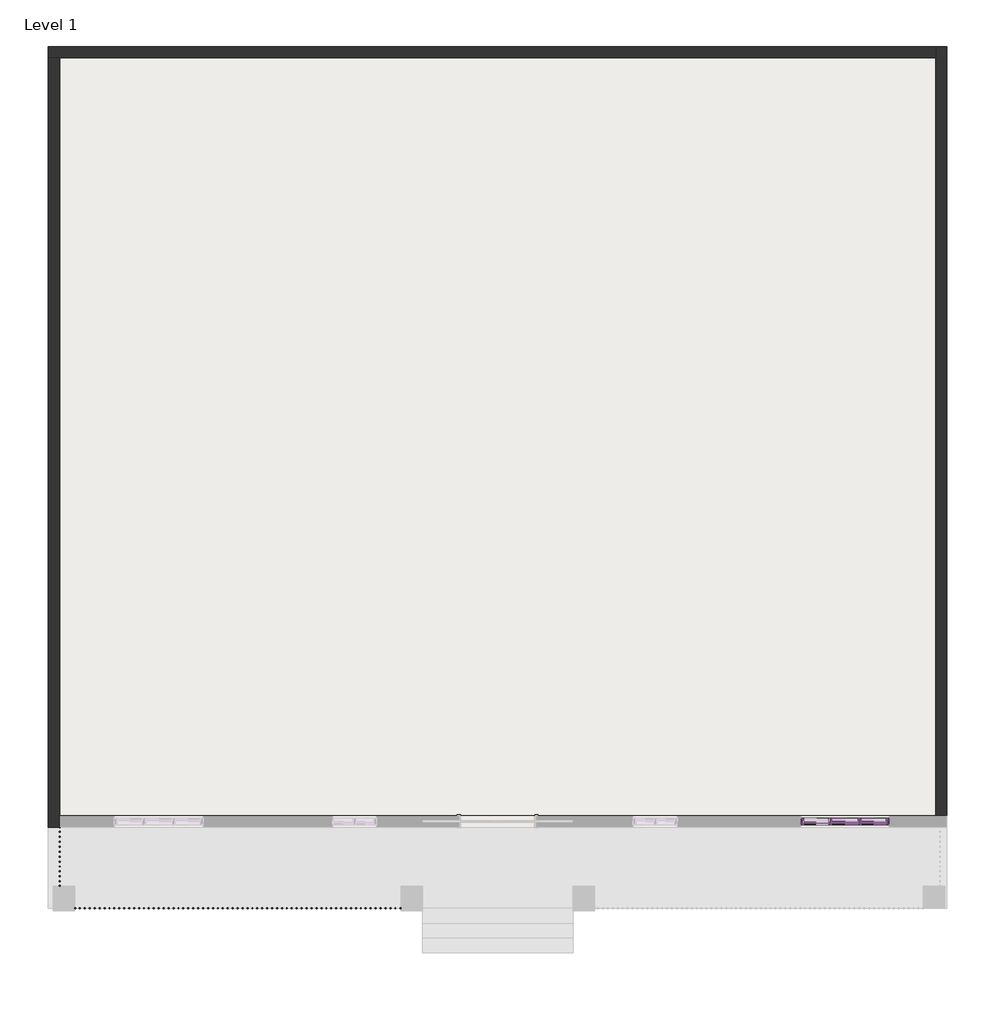
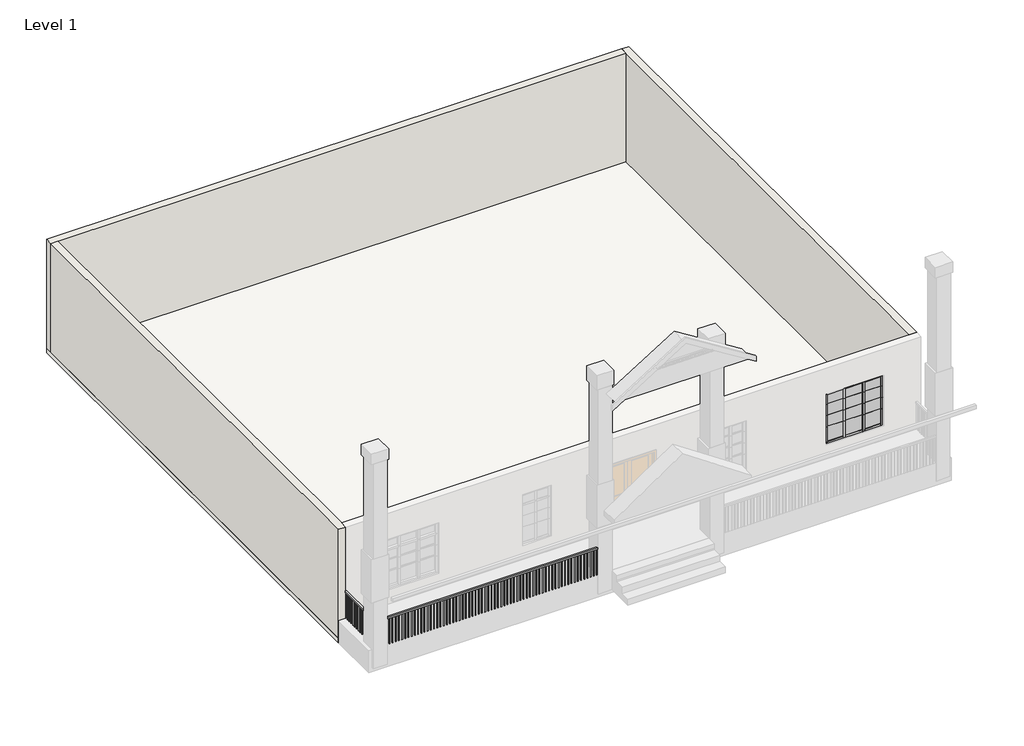
# One storey, part 2 of 3: 27 members, 12 plates, 3 walls, 2 railings, 1 slab.
"""IFC4 building model written with IfcOpenShell, lengths in millimetres."""

from ifc_helpers import new_model, si_unit, frame, origin, place, context, project, spatial, polyline, outline, extrude, faceted_brep, transform, mapped, element, save
from components import member_9625144b, member_80fbcd94, member_0b7646a3, member_bc554fa6, member_a980948f, member_03a502dc, member_dfe75557, member_50cacee6, system_panel_glazed_6026b5c4, system_panel_glazed_0f474f61, system_panel_glazed_969e6b50, system_panel_glazed_86de8a05, system_panel_glazed_f6df7fa7, system_panel_glazed_f12bf2b5

model = new_model("IFC4")

# Units and contexts
model_context = context("Model", 3, world=origin())
ifc_project = project(units=[si_unit("LENGTHUNIT", "METRE", prefix="MILLI")], contexts=[model_context])

# Site, building, storey
site = spatial("IfcSite", under=ifc_project)
building = spatial("IfcBuilding", under=site)
storey = spatial("IfcBuildingStorey", under=building, Name="Level 1", Elevation=0.0)

# Members
placement = place(None, origin())
member_shape = member_9625144b(model_context)
element("IfcMember", 1, ObjectType="Rectangular Mullion : 1\" Square", at=placement, inside=storey, context=model_context, shape_type="MappedRepresentation", body=[
    mapped(member_shape, transform((6987.2079341, -6986.1878342, 2006.6), x_axis=(0.0, 0.0, 1.0), y_axis=(0.0, 1.0, 0.0), z_axis=(-1.0, 0.0, 0.0))),
])
element("IfcMember", 2, ObjectType="Rectangular Mullion : 1\" Square", at=placement, inside=storey, context=model_context, shape_type="MappedRepresentation", body=[
    mapped(member_shape, transform((6987.2079341, -6986.1878342, 1625.6), x_axis=(0.0, 0.0, 1.0), y_axis=(0.0, 1.0, 0.0), z_axis=(-1.0, 0.0, 0.0))),
])
element("IfcMember", 3, ObjectType="Rectangular Mullion : 1\" Square", at=placement, inside=storey, context=model_context, shape_type="MappedRepresentation", body=[
    mapped(member_shape, transform((6987.2079341, -6986.1878342, 2387.6), x_axis=(0.0, 0.0, 1.0), y_axis=(0.0, 1.0, 0.0), z_axis=(-1.0, 0.0, 0.0))),
])
member_2_shape = member_80fbcd94(model_context)
element("IfcMember", 4, ObjectType="Rectangular Mullion : 1\" Square", at=placement, inside=storey, context=model_context, shape_type="MappedRepresentation", body=[
    mapped(member_2_shape, transform((6377.6079341, -6986.1878342, 2006.6), x_axis=(0.0, 0.0, 1.0), y_axis=(0.0, 1.0, 0.0), z_axis=(-1.0, 0.0, 0.0))),
])
element("IfcMember", 5, ObjectType="Rectangular Mullion : 1\" Square", at=placement, inside=storey, context=model_context, shape_type="MappedRepresentation", body=[
    mapped(member_2_shape, transform((6377.6079341, -6986.1878342, 1625.6), x_axis=(0.0, 0.0, 1.0), y_axis=(0.0, 1.0, 0.0), z_axis=(-1.0, 0.0, 0.0))),
])
element("IfcMember", 6, ObjectType="Rectangular Mullion : 1\" Square", at=placement, inside=storey, context=model_context, shape_type="MappedRepresentation", body=[
    mapped(member_2_shape, transform((6377.6079341, -6986.1878342, 2387.6), x_axis=(0.0, 0.0, 1.0), y_axis=(0.0, 1.0, 0.0), z_axis=(-1.0, 0.0, 0.0))),
])
member_3_shape = member_0b7646a3(model_context)
element("IfcMember", 7, ObjectType="Rectangular Mullion : 2.5\" x 5\" rectangular", at=placement, inside=storey, context=model_context, shape_type="MappedRepresentation", body=[
    mapped(member_3_shape, transform((6987.2079341, -6986.1878342, 2768.6), x_axis=(0.0, 0.0, 1.0), y_axis=(0.0, 1.0, 0.0), z_axis=(-1.0, 0.0, 0.0))),
])
element("IfcMember", 8, ObjectType="Rectangular Mullion : 2.5\" x 5\" rectangular", at=placement, inside=storey, context=model_context, shape_type="MappedRepresentation", body=[
    mapped(member_3_shape, transform((7501.5579341, -6986.1878342, 1066.8), x_axis=(0.0, 0.0, -1.0), y_axis=(0.0, 1.0, 0.0), z_axis=(1.0, 0.0, 0.0))),
])
element("IfcMember", 9, ObjectType="Rectangular Mullion : 2.5\" x 5\" rectangular", at=placement, inside=storey, context=model_context, shape_type="MappedRepresentation", body=[
    mapped(member_3_shape, transform((6314.1079341, -6986.1878342, 1066.8), x_axis=(0.0, 0.0, -1.0), y_axis=(0.0, 1.0, 0.0), z_axis=(1.0, 0.0, 0.0))),
])
member_4_shape = member_bc554fa6(model_context)
element("IfcMember", 10, ObjectType="Rectangular Mullion : 2.5\" x 5\" rectangular", at=placement, inside=storey, context=model_context, shape_type="MappedRepresentation", body=[
    mapped(member_4_shape, transform((6345.8579341, -6986.1878342, 1066.8), x_axis=(-1.0, 0.0, 0.0), y_axis=(0.0, 1.0, 0.0), z_axis=(0.0, 0.0, -1.0))),
])
element("IfcMember", 11, ObjectType="Rectangular Mullion : 2.5\" x 5\" rectangular", at=placement, inside=storey, context=model_context, shape_type="MappedRepresentation", body=[
    mapped(member_4_shape, transform((6955.4579341, -6986.1878342, 1066.8), x_axis=(-1.0, 0.0, 0.0), y_axis=(0.0, 1.0, 0.0), z_axis=(0.0, 0.0, -1.0))),
])
member_5_shape = member_a980948f(model_context)
element("IfcMember", 12, ObjectType="Rectangular Mullion : 2.5\" x 5\" rectangular", at=placement, inside=storey, context=model_context, shape_type="MappedRepresentation", body=[
    mapped(member_5_shape, transform((6923.7079341, -6986.1878342, 1066.8), x_axis=(0.0, 0.0, -1.0), y_axis=(0.0, 1.0, 0.0), z_axis=(1.0, 0.0, 0.0))),
])
element("IfcMember", 13, ObjectType="Rectangular Mullion : 2.5\" x 5\" rectangular", at=placement, inside=storey, context=model_context, shape_type="MappedRepresentation", body=[
    mapped(member_5_shape, transform((6377.6079341, -6986.1878342, 2768.6), x_axis=(0.0, 0.0, 1.0), y_axis=(0.0, 1.0, 0.0), z_axis=(-1.0, 0.0, 0.0))),
])
member_6_shape = member_03a502dc(model_context)
element("IfcMember", 14, ObjectType="Rectangular Mullion : 2.5\" x 5\" rectangular", at=placement, inside=storey, context=model_context, shape_type="MappedRepresentation", body=[
    mapped(member_6_shape, transform((6345.8579341, -6986.1878342, 2387.6), x_axis=(-1.0, 0.0, 0.0), y_axis=(0.0, 1.0, 0.0), z_axis=(0.0, 0.0, -1.0))),
])
element("IfcMember", 15, ObjectType="Rectangular Mullion : 2.5\" x 5\" rectangular", at=placement, inside=storey, context=model_context, shape_type="MappedRepresentation", body=[
    mapped(member_6_shape, transform((6955.4579341, -6986.1878342, 2387.6), x_axis=(-1.0, 0.0, 0.0), y_axis=(0.0, 1.0, 0.0), z_axis=(0.0, 0.0, -1.0))),
])
element("IfcMember", 16, ObjectType="Rectangular Mullion : 2.5\" x 5\" rectangular", at=placement, inside=storey, context=model_context, shape_type="MappedRepresentation", body=[
    mapped(member_6_shape, transform((6345.8579341, -6986.1878342, 2006.6), x_axis=(-1.0, 0.0, 0.0), y_axis=(0.0, 1.0, 0.0), z_axis=(0.0, 0.0, -1.0))),
])
element("IfcMember", 17, ObjectType="Rectangular Mullion : 2.5\" x 5\" rectangular", at=placement, inside=storey, context=model_context, shape_type="MappedRepresentation", body=[
    mapped(member_6_shape, transform((6345.8579341, -6986.1878342, 1625.6), x_axis=(-1.0, 0.0, 0.0), y_axis=(0.0, 1.0, 0.0), z_axis=(0.0, 0.0, -1.0))),
])
element("IfcMember", 18, ObjectType="Rectangular Mullion : 2.5\" x 5\" rectangular", at=placement, inside=storey, context=model_context, shape_type="MappedRepresentation", body=[
    mapped(member_6_shape, transform((6955.4579341, -6986.1878342, 2006.6), x_axis=(-1.0, 0.0, 0.0), y_axis=(0.0, 1.0, 0.0), z_axis=(0.0, 0.0, -1.0))),
])
element("IfcMember", 19, ObjectType="Rectangular Mullion : 2.5\" x 5\" rectangular", at=placement, inside=storey, context=model_context, shape_type="MappedRepresentation", body=[
    mapped(member_6_shape, transform((6955.4579341, -6986.1878342, 1625.6), x_axis=(-1.0, 0.0, 0.0), y_axis=(0.0, 1.0, 0.0), z_axis=(0.0, 0.0, -1.0))),
])
member_7_shape = member_dfe75557(model_context)
element("IfcMember", 20, ObjectType="Rectangular Mullion : 2.5\" x 5\" rectangular", at=placement, inside=storey, context=model_context, shape_type="MappedRepresentation", body=[
    mapped(member_7_shape, transform((7565.0579341, -6986.1878342, 2768.6), x_axis=(1.0, 0.0, 0.0), y_axis=(0.0, 1.0, 0.0), z_axis=(0.0, 0.0, 1.0))),
])
member_8_shape = member_50cacee6(model_context)
element("IfcMember", 21, ObjectType="Rectangular Mullion : 2.5\" x 5\" rectangular", at=placement, inside=storey, context=model_context, shape_type="MappedRepresentation", body=[
    mapped(member_8_shape, transform((5736.2579341, -6986.1878342, 1066.8), x_axis=(-1.0, 0.0, 0.0), y_axis=(0.0, 1.0, 0.0), z_axis=(0.0, 0.0, -1.0))),
])
element("IfcMember", 22, ObjectType="Rectangular Mullion : 2.5\" x 5\" rectangular", at=placement, inside=storey, context=model_context, shape_type="MappedRepresentation", body=[
    mapped(member_7_shape, transform((5736.2579341, -6986.1878342, 2387.6), x_axis=(-1.0, 0.0, 0.0), y_axis=(0.0, 1.0, 0.0), z_axis=(0.0, 0.0, -1.0))),
])
element("IfcMember", 23, ObjectType="Rectangular Mullion : 2.5\" x 5\" rectangular", at=placement, inside=storey, context=model_context, shape_type="MappedRepresentation", body=[
    mapped(member_7_shape, transform((5736.2579341, -6986.1878342, 2006.6), x_axis=(-1.0, 0.0, 0.0), y_axis=(0.0, 1.0, 0.0), z_axis=(0.0, 0.0, -1.0))),
])
element("IfcMember", 24, ObjectType="Rectangular Mullion : 2.5\" x 5\" rectangular", at=placement, inside=storey, context=model_context, shape_type="MappedRepresentation", body=[
    mapped(member_7_shape, transform((5736.2579341, -6986.1878342, 1625.6), x_axis=(-1.0, 0.0, 0.0), y_axis=(0.0, 1.0, 0.0), z_axis=(0.0, 0.0, -1.0))),
])
element("IfcMember", 25, ObjectType="Rectangular Mullion : 2.5\" x 5\" rectangular", at=placement, inside=storey, context=model_context, shape_type="MappedRepresentation", body=[
    mapped(member_7_shape, transform((7565.0579341, -6986.1878342, 2387.6), x_axis=(1.0, 0.0, 0.0), y_axis=(0.0, 1.0, 0.0), z_axis=(0.0, 0.0, 1.0))),
])
element("IfcMember", 26, ObjectType="Rectangular Mullion : 2.5\" x 5\" rectangular", at=placement, inside=storey, context=model_context, shape_type="MappedRepresentation", body=[
    mapped(member_7_shape, transform((7565.0579341, -6986.1878342, 2006.6), x_axis=(1.0, 0.0, 0.0), y_axis=(0.0, 1.0, 0.0), z_axis=(0.0, 0.0, 1.0))),
])
element("IfcMember", 27, ObjectType="Rectangular Mullion : 2.5\" x 5\" rectangular", at=placement, inside=storey, context=model_context, shape_type="MappedRepresentation", body=[
    mapped(member_8_shape, transform((7565.0579341, -6986.1878342, 1625.6), x_axis=(1.0, 0.0, 0.0), y_axis=(0.0, 1.0, 0.0), z_axis=(0.0, 0.0, 1.0))),
])

# Plates
system_panel_glazed_shape = system_panel_glazed_6026b5c4(model_context)
element("IfcPlate", 28, ObjectType="System Panel : Glazed", at=placement, inside=storey, context=model_context, shape_type="MappedRepresentation", body=[
    mapped(system_panel_glazed_shape, transform((7244.3829341, -6986.1878342, 1130.3), x_axis=(-1.0, 0.0, 0.0), y_axis=(0.0, -1.0, 0.0), z_axis=(0.0, 0.0, 1.0))),
])
element("IfcPlate", 29, ObjectType="System Panel : Glazed", at=placement, inside=storey, context=model_context, shape_type="MappedRepresentation", body=[
    mapped(system_panel_glazed_shape, transform((6056.9329341, -6986.1878342, 1130.3), x_axis=(-1.0, 0.0, 0.0), y_axis=(0.0, -1.0, 0.0), z_axis=(0.0, 0.0, 1.0))),
])
system_panel_glazed_2_shape = system_panel_glazed_0f474f61(model_context)
element("IfcPlate", 30, ObjectType="System Panel : Glazed", at=placement, inside=storey, context=model_context, shape_type="MappedRepresentation", body=[
    mapped(system_panel_glazed_2_shape, transform((6650.6579341, -6986.1878342, 1130.3), x_axis=(-1.0, 0.0, 0.0), y_axis=(0.0, -1.0, 0.0), z_axis=(0.0, 0.0, 1.0))),
])
system_panel_glazed_3_shape = system_panel_glazed_969e6b50(model_context)
element("IfcPlate", 31, ObjectType="System Panel : Glazed", at=placement, inside=storey, context=model_context, shape_type="MappedRepresentation", body=[
    mapped(system_panel_glazed_3_shape, transform((7244.3829341, -6986.1878342, 2006.6), x_axis=(-1.0, 0.0, 0.0), y_axis=(0.0, -1.0, 0.0), z_axis=(0.0, 0.0, 1.0))),
])
element("IfcPlate", 32, ObjectType="System Panel : Glazed", at=placement, inside=storey, context=model_context, shape_type="MappedRepresentation", body=[
    mapped(system_panel_glazed_3_shape, transform((6056.9329341, -6986.1878342, 2006.6), x_axis=(-1.0, 0.0, 0.0), y_axis=(0.0, -1.0, 0.0), z_axis=(0.0, 0.0, 1.0))),
])
element("IfcPlate", 33, ObjectType="System Panel : Glazed", at=placement, inside=storey, context=model_context, shape_type="MappedRepresentation", body=[
    mapped(system_panel_glazed_3_shape, transform((7244.3829341, -6986.1878342, 1625.6), x_axis=(-1.0, 0.0, 0.0), y_axis=(0.0, -1.0, 0.0), z_axis=(0.0, 0.0, 1.0))),
])
element("IfcPlate", 34, ObjectType="System Panel : Glazed", at=placement, inside=storey, context=model_context, shape_type="MappedRepresentation", body=[
    mapped(system_panel_glazed_3_shape, transform((6056.9329341, -6986.1878342, 1625.6), x_axis=(-1.0, 0.0, 0.0), y_axis=(0.0, -1.0, 0.0), z_axis=(0.0, 0.0, 1.0))),
])
system_panel_glazed_4_shape = system_panel_glazed_86de8a05(model_context)
element("IfcPlate", 35, ObjectType="System Panel : Glazed", at=placement, inside=storey, context=model_context, shape_type="MappedRepresentation", body=[
    mapped(system_panel_glazed_4_shape, transform((6650.6579341, -6986.1878342, 2006.6), x_axis=(-1.0, 0.0, 0.0), y_axis=(0.0, -1.0, 0.0), z_axis=(0.0, 0.0, 1.0))),
])
element("IfcPlate", 36, ObjectType="System Panel : Glazed", at=placement, inside=storey, context=model_context, shape_type="MappedRepresentation", body=[
    mapped(system_panel_glazed_4_shape, transform((6650.6579341, -6986.1878342, 1625.6), x_axis=(-1.0, 0.0, 0.0), y_axis=(0.0, -1.0, 0.0), z_axis=(0.0, 0.0, 1.0))),
])
system_panel_glazed_5_shape = system_panel_glazed_f6df7fa7(model_context)
element("IfcPlate", 37, ObjectType="System Panel : Glazed", at=placement, inside=storey, context=model_context, shape_type="MappedRepresentation", body=[
    mapped(system_panel_glazed_5_shape, transform((7244.3829341, -6986.1878342, 2387.6), x_axis=(-1.0, 0.0, 0.0), y_axis=(0.0, -1.0, 0.0), z_axis=(0.0, 0.0, 1.0))),
])
element("IfcPlate", 38, ObjectType="System Panel : Glazed", at=placement, inside=storey, context=model_context, shape_type="MappedRepresentation", body=[
    mapped(system_panel_glazed_5_shape, transform((6056.9329341, -6986.1878342, 2387.6), x_axis=(-1.0, 0.0, 0.0), y_axis=(0.0, -1.0, 0.0), z_axis=(0.0, 0.0, 1.0))),
])
system_panel_glazed_6_shape = system_panel_glazed_f12bf2b5(model_context)
element("IfcPlate", 39, ObjectType="System Panel : Glazed", at=placement, inside=storey, context=model_context, shape_type="MappedRepresentation", body=[
    mapped(system_panel_glazed_6_shape, transform((6650.6579341, -6986.1878342, 2387.6), x_axis=(-1.0, 0.0, 0.0), y_axis=(0.0, -1.0, 0.0), z_axis=(0.0, 0.0, 1.0))),
])

# Railings
element("IfcRailing", 40, ObjectType="Handrail - Rectangular", at=placement, inside=storey, context=model_context, shape_type="SweptSolid", body=[
    extrude(outline(polyline([(-9224.3420659, -8800.5902135), (-9224.3420659, -8749.7902135), (-2506.0420659, -8749.7902135), (-2506.0420659, -8800.5902135), (-9224.3420659, -8800.5902135)])), frame((0.0, 0.0, 1473.2), z_axis=(0.0, 0.0, 1.0), x_axis=(1.0, 0.0, 0.0)), (0.0, 0.0, 1.0), 50.8),
    extrude(outline(polyline([(-2528.2670659, -8784.7152135), (-2528.2670659, -8765.6652135), (-2509.2170659, -8765.6652135), (-2509.2170659, -8784.7152135), (-2528.2670659, -8784.7152135)])), frame((0.0, 0.0, 609.6), z_axis=(0.0, 0.0, 1.0), x_axis=(1.0, 0.0, 0.0)), (0.0, 0.0, 1.0), 863.6),
    extrude(outline(polyline([(-2629.8670659, -8784.7152135), (-2629.8670659, -8765.6652135), (-2610.8170659, -8765.6652135), (-2610.8170659, -8784.7152135), (-2629.8670659, -8784.7152135)])), frame((0.0, 0.0, 609.6), z_axis=(0.0, 0.0, 1.0), x_axis=(1.0, 0.0, 0.0)), (0.0, 0.0, 1.0), 863.6),
    extrude(outline(polyline([(-2731.4670659, -8784.7152135), (-2731.4670659, -8765.6652135), (-2712.4170659, -8765.6652135), (-2712.4170659, -8784.7152135), (-2731.4670659, -8784.7152135)])), frame((0.0, 0.0, 609.6), z_axis=(0.0, 0.0, 1.0), x_axis=(1.0, 0.0, 0.0)), (0.0, 0.0, 1.0), 863.6),
    extrude(outline(polyline([(-2833.0670659, -8784.7152135), (-2833.0670659, -8765.6652135), (-2814.0170659, -8765.6652135), (-2814.0170659, -8784.7152135), (-2833.0670659, -8784.7152135)])), frame((0.0, 0.0, 609.6), z_axis=(0.0, 0.0, 1.0), x_axis=(1.0, 0.0, 0.0)), (0.0, 0.0, 1.0), 863.6),
    extrude(outline(polyline([(-2934.6670659, -8784.7152135), (-2934.6670659, -8765.6652135), (-2915.6170659, -8765.6652135), (-2915.6170659, -8784.7152135), (-2934.6670659, -8784.7152135)])), frame((0.0, 0.0, 609.6), z_axis=(0.0, 0.0, 1.0), x_axis=(1.0, 0.0, 0.0)), (0.0, 0.0, 1.0), 863.6),
    extrude(outline(polyline([(-3036.2670659, -8784.7152135), (-3036.2670659, -8765.6652135), (-3017.2170659, -8765.6652135), (-3017.2170659, -8784.7152135), (-3036.2670659, -8784.7152135)])), frame((0.0, 0.0, 609.6), z_axis=(0.0, 0.0, 1.0), x_axis=(1.0, 0.0, 0.0)), (0.0, 0.0, 1.0), 863.6),
    extrude(outline(polyline([(-3137.8670659, -8784.7152135), (-3137.8670659, -8765.6652135), (-3118.8170659, -8765.6652135), (-3118.8170659, -8784.7152135), (-3137.8670659, -8784.7152135)])), frame((0.0, 0.0, 609.6), z_axis=(0.0, 0.0, 1.0), x_axis=(1.0, 0.0, 0.0)), (0.0, 0.0, 1.0), 863.6),
    extrude(outline(polyline([(-3239.4670659, -8784.7152135), (-3239.4670659, -8765.6652135), (-3220.4170659, -8765.6652135), (-3220.4170659, -8784.7152135), (-3239.4670659, -8784.7152135)])), frame((0.0, 0.0, 609.6), z_axis=(0.0, 0.0, 1.0), x_axis=(1.0, 0.0, 0.0)), (0.0, 0.0, 1.0), 863.6),
    extrude(outline(polyline([(-3341.0670659, -8784.7152135), (-3341.0670659, -8765.6652135), (-3322.0170659, -8765.6652135), (-3322.0170659, -8784.7152135), (-3341.0670659, -8784.7152135)])), frame((0.0, 0.0, 609.6), z_axis=(0.0, 0.0, 1.0), x_axis=(1.0, 0.0, 0.0)), (0.0, 0.0, 1.0), 863.6),
    extrude(outline(polyline([(-3442.6670659, -8784.7152135), (-3442.6670659, -8765.6652135), (-3423.6170659, -8765.6652135), (-3423.6170659, -8784.7152135), (-3442.6670659, -8784.7152135)])), frame((0.0, 0.0, 609.6), z_axis=(0.0, 0.0, 1.0), x_axis=(1.0, 0.0, 0.0)), (0.0, 0.0, 1.0), 863.6),
    extrude(outline(polyline([(-3544.2670659, -8784.7152135), (-3544.2670659, -8765.6652135), (-3525.2170659, -8765.6652135), (-3525.2170659, -8784.7152135), (-3544.2670659, -8784.7152135)])), frame((0.0, 0.0, 609.6), z_axis=(0.0, 0.0, 1.0), x_axis=(1.0, 0.0, 0.0)), (0.0, 0.0, 1.0), 863.6),
    extrude(outline(polyline([(-3645.8670659, -8784.7152135), (-3645.8670659, -8765.6652135), (-3626.8170659, -8765.6652135), (-3626.8170659, -8784.7152135), (-3645.8670659, -8784.7152135)])), frame((0.0, 0.0, 609.6), z_axis=(0.0, 0.0, 1.0), x_axis=(1.0, 0.0, 0.0)), (0.0, 0.0, 1.0), 863.6),
    extrude(outline(polyline([(-3747.4670659, -8784.7152135), (-3747.4670659, -8765.6652135), (-3728.4170659, -8765.6652135), (-3728.4170659, -8784.7152135), (-3747.4670659, -8784.7152135)])), frame((0.0, 0.0, 609.6), z_axis=(0.0, 0.0, 1.0), x_axis=(1.0, 0.0, 0.0)), (0.0, 0.0, 1.0), 863.6),
    extrude(outline(polyline([(-3849.0670659, -8784.7152135), (-3849.0670659, -8765.6652135), (-3830.0170659, -8765.6652135), (-3830.0170659, -8784.7152135), (-3849.0670659, -8784.7152135)])), frame((0.0, 0.0, 609.6), z_axis=(0.0, 0.0, 1.0), x_axis=(1.0, 0.0, 0.0)), (0.0, 0.0, 1.0), 863.6),
    extrude(outline(polyline([(-3950.6670659, -8784.7152135), (-3950.6670659, -8765.6652135), (-3931.6170659, -8765.6652135), (-3931.6170659, -8784.7152135), (-3950.6670659, -8784.7152135)])), frame((0.0, 0.0, 609.6), z_axis=(0.0, 0.0, 1.0), x_axis=(1.0, 0.0, 0.0)), (0.0, 0.0, 1.0), 863.6),
    extrude(outline(polyline([(-4052.2670659, -8784.7152135), (-4052.2670659, -8765.6652135), (-4033.2170659, -8765.6652135), (-4033.2170659, -8784.7152135), (-4052.2670659, -8784.7152135)])), frame((0.0, 0.0, 609.6), z_axis=(0.0, 0.0, 1.0), x_axis=(1.0, 0.0, 0.0)), (0.0, 0.0, 1.0), 863.6),
    extrude(outline(polyline([(-4153.8670659, -8784.7152135), (-4153.8670659, -8765.6652135), (-4134.8170659, -8765.6652135), (-4134.8170659, -8784.7152135), (-4153.8670659, -8784.7152135)])), frame((0.0, 0.0, 609.6), z_axis=(0.0, 0.0, 1.0), x_axis=(1.0, 0.0, 0.0)), (0.0, 0.0, 1.0), 863.6),
    extrude(outline(polyline([(-4255.4670659, -8784.7152135), (-4255.4670659, -8765.6652135), (-4236.4170659, -8765.6652135), (-4236.4170659, -8784.7152135), (-4255.4670659, -8784.7152135)])), frame((0.0, 0.0, 609.6), z_axis=(0.0, 0.0, 1.0), x_axis=(1.0, 0.0, 0.0)), (0.0, 0.0, 1.0), 863.6),
    extrude(outline(polyline([(-4357.0670659, -8784.7152135), (-4357.0670659, -8765.6652135), (-4338.0170659, -8765.6652135), (-4338.0170659, -8784.7152135), (-4357.0670659, -8784.7152135)])), frame((0.0, 0.0, 609.6), z_axis=(0.0, 0.0, 1.0), x_axis=(1.0, 0.0, 0.0)), (0.0, 0.0, 1.0), 863.6),
    extrude(outline(polyline([(-4458.6670659, -8784.7152135), (-4458.6670659, -8765.6652135), (-4439.6170659, -8765.6652135), (-4439.6170659, -8784.7152135), (-4458.6670659, -8784.7152135)])), frame((0.0, 0.0, 609.6), z_axis=(0.0, 0.0, 1.0), x_axis=(1.0, 0.0, 0.0)), (0.0, 0.0, 1.0), 863.6),
    extrude(outline(polyline([(-4560.2670659, -8784.7152135), (-4560.2670659, -8765.6652135), (-4541.2170659, -8765.6652135), (-4541.2170659, -8784.7152135), (-4560.2670659, -8784.7152135)])), frame((0.0, 0.0, 609.6), z_axis=(0.0, 0.0, 1.0), x_axis=(1.0, 0.0, 0.0)), (0.0, 0.0, 1.0), 863.6),
    extrude(outline(polyline([(-4661.8670659, -8784.7152135), (-4661.8670659, -8765.6652135), (-4642.8170659, -8765.6652135), (-4642.8170659, -8784.7152135), (-4661.8670659, -8784.7152135)])), frame((0.0, 0.0, 609.6), z_axis=(0.0, 0.0, 1.0), x_axis=(1.0, 0.0, 0.0)), (0.0, 0.0, 1.0), 863.6),
    extrude(outline(polyline([(-4763.4670659, -8784.7152135), (-4763.4670659, -8765.6652135), (-4744.4170659, -8765.6652135), (-4744.4170659, -8784.7152135), (-4763.4670659, -8784.7152135)])), frame((0.0, 0.0, 609.6), z_axis=(0.0, 0.0, 1.0), x_axis=(1.0, 0.0, 0.0)), (0.0, 0.0, 1.0), 863.6),
    extrude(outline(polyline([(-4865.0670659, -8784.7152135), (-4865.0670659, -8765.6652135), (-4846.0170659, -8765.6652135), (-4846.0170659, -8784.7152135), (-4865.0670659, -8784.7152135)])), frame((0.0, 0.0, 609.6), z_axis=(0.0, 0.0, 1.0), x_axis=(1.0, 0.0, 0.0)), (0.0, 0.0, 1.0), 863.6),
    extrude(outline(polyline([(-4966.6670659, -8784.7152135), (-4966.6670659, -8765.6652135), (-4947.6170659, -8765.6652135), (-4947.6170659, -8784.7152135), (-4966.6670659, -8784.7152135)])), frame((0.0, 0.0, 609.6), z_axis=(0.0, 0.0, 1.0), x_axis=(1.0, 0.0, 0.0)), (0.0, 0.0, 1.0), 863.6),
    extrude(outline(polyline([(-5068.2670659, -8784.7152135), (-5068.2670659, -8765.6652135), (-5049.2170659, -8765.6652135), (-5049.2170659, -8784.7152135), (-5068.2670659, -8784.7152135)])), frame((0.0, 0.0, 609.6), z_axis=(0.0, 0.0, 1.0), x_axis=(1.0, 0.0, 0.0)), (0.0, 0.0, 1.0), 863.6),
    extrude(outline(polyline([(-5169.8670659, -8784.7152135), (-5169.8670659, -8765.6652135), (-5150.8170659, -8765.6652135), (-5150.8170659, -8784.7152135), (-5169.8670659, -8784.7152135)])), frame((0.0, 0.0, 609.6), z_axis=(0.0, 0.0, 1.0), x_axis=(1.0, 0.0, 0.0)), (0.0, 0.0, 1.0), 863.6),
    extrude(outline(polyline([(-5271.4670659, -8784.7152135), (-5271.4670659, -8765.6652135), (-5252.4170659, -8765.6652135), (-5252.4170659, -8784.7152135), (-5271.4670659, -8784.7152135)])), frame((0.0, 0.0, 609.6), z_axis=(0.0, 0.0, 1.0), x_axis=(1.0, 0.0, 0.0)), (0.0, 0.0, 1.0), 863.6),
    extrude(outline(polyline([(-5373.0670659, -8784.7152135), (-5373.0670659, -8765.6652135), (-5354.0170659, -8765.6652135), (-5354.0170659, -8784.7152135), (-5373.0670659, -8784.7152135)])), frame((0.0, 0.0, 609.6), z_axis=(0.0, 0.0, 1.0), x_axis=(1.0, 0.0, 0.0)), (0.0, 0.0, 1.0), 863.6),
    extrude(outline(polyline([(-5474.6670659, -8784.7152135), (-5474.6670659, -8765.6652135), (-5455.6170659, -8765.6652135), (-5455.6170659, -8784.7152135), (-5474.6670659, -8784.7152135)])), frame((0.0, 0.0, 609.6), z_axis=(0.0, 0.0, 1.0), x_axis=(1.0, 0.0, 0.0)), (0.0, 0.0, 1.0), 863.6),
    extrude(outline(polyline([(-5576.2670659, -8784.7152135), (-5576.2670659, -8765.6652135), (-5557.2170659, -8765.6652135), (-5557.2170659, -8784.7152135), (-5576.2670659, -8784.7152135)])), frame((0.0, 0.0, 609.6), z_axis=(0.0, 0.0, 1.0), x_axis=(1.0, 0.0, 0.0)), (0.0, 0.0, 1.0), 863.6),
    extrude(outline(polyline([(-5677.8670659, -8784.7152135), (-5677.8670659, -8765.6652135), (-5658.8170659, -8765.6652135), (-5658.8170659, -8784.7152135), (-5677.8670659, -8784.7152135)])), frame((0.0, 0.0, 609.6), z_axis=(0.0, 0.0, 1.0), x_axis=(1.0, 0.0, 0.0)), (0.0, 0.0, 1.0), 863.6),
    extrude(outline(polyline([(-5779.4670659, -8784.7152135), (-5779.4670659, -8765.6652135), (-5760.4170659, -8765.6652135), (-5760.4170659, -8784.7152135), (-5779.4670659, -8784.7152135)])), frame((0.0, 0.0, 609.6), z_axis=(0.0, 0.0, 1.0), x_axis=(1.0, 0.0, 0.0)), (0.0, 0.0, 1.0), 863.6),
    extrude(outline(polyline([(-5881.0670659, -8784.7152135), (-5881.0670659, -8765.6652135), (-5862.0170659, -8765.6652135), (-5862.0170659, -8784.7152135), (-5881.0670659, -8784.7152135)])), frame((0.0, 0.0, 609.6), z_axis=(0.0, 0.0, 1.0), x_axis=(1.0, 0.0, 0.0)), (0.0, 0.0, 1.0), 863.6),
    extrude(outline(polyline([(-5982.6670659, -8784.7152135), (-5982.6670659, -8765.6652135), (-5963.6170659, -8765.6652135), (-5963.6170659, -8784.7152135), (-5982.6670659, -8784.7152135)])), frame((0.0, 0.0, 609.6), z_axis=(0.0, 0.0, 1.0), x_axis=(1.0, 0.0, 0.0)), (0.0, 0.0, 1.0), 863.6),
    extrude(outline(polyline([(-6084.2670659, -8784.7152135), (-6084.2670659, -8765.6652135), (-6065.2170659, -8765.6652135), (-6065.2170659, -8784.7152135), (-6084.2670659, -8784.7152135)])), frame((0.0, 0.0, 609.6), z_axis=(0.0, 0.0, 1.0), x_axis=(1.0, 0.0, 0.0)), (0.0, 0.0, 1.0), 863.6),
    extrude(outline(polyline([(-6185.8670659, -8784.7152135), (-6185.8670659, -8765.6652135), (-6166.8170659, -8765.6652135), (-6166.8170659, -8784.7152135), (-6185.8670659, -8784.7152135)])), frame((0.0, 0.0, 609.6), z_axis=(0.0, 0.0, 1.0), x_axis=(1.0, 0.0, 0.0)), (0.0, 0.0, 1.0), 863.6),
    extrude(outline(polyline([(-6287.4670659, -8784.7152135), (-6287.4670659, -8765.6652135), (-6268.4170659, -8765.6652135), (-6268.4170659, -8784.7152135), (-6287.4670659, -8784.7152135)])), frame((0.0, 0.0, 609.6), z_axis=(0.0, 0.0, 1.0), x_axis=(1.0, 0.0, 0.0)), (0.0, 0.0, 1.0), 863.6),
    extrude(outline(polyline([(-6389.0670659, -8784.7152135), (-6389.0670659, -8765.6652135), (-6370.0170659, -8765.6652135), (-6370.0170659, -8784.7152135), (-6389.0670659, -8784.7152135)])), frame((0.0, 0.0, 609.6), z_axis=(0.0, 0.0, 1.0), x_axis=(1.0, 0.0, 0.0)), (0.0, 0.0, 1.0), 863.6),
    extrude(outline(polyline([(-6490.6670659, -8784.7152135), (-6490.6670659, -8765.6652135), (-6471.6170659, -8765.6652135), (-6471.6170659, -8784.7152135), (-6490.6670659, -8784.7152135)])), frame((0.0, 0.0, 609.6), z_axis=(0.0, 0.0, 1.0), x_axis=(1.0, 0.0, 0.0)), (0.0, 0.0, 1.0), 863.6),
    extrude(outline(polyline([(-6592.2670659, -8784.7152135), (-6592.2670659, -8765.6652135), (-6573.2170659, -8765.6652135), (-6573.2170659, -8784.7152135), (-6592.2670659, -8784.7152135)])), frame((0.0, 0.0, 609.6), z_axis=(0.0, 0.0, 1.0), x_axis=(1.0, 0.0, 0.0)), (0.0, 0.0, 1.0), 863.6),
    extrude(outline(polyline([(-6693.8670659, -8784.7152135), (-6693.8670659, -8765.6652135), (-6674.8170659, -8765.6652135), (-6674.8170659, -8784.7152135), (-6693.8670659, -8784.7152135)])), frame((0.0, 0.0, 609.6), z_axis=(0.0, 0.0, 1.0), x_axis=(1.0, 0.0, 0.0)), (0.0, 0.0, 1.0), 863.6),
    extrude(outline(polyline([(-6795.4670659, -8784.7152135), (-6795.4670659, -8765.6652135), (-6776.4170659, -8765.6652135), (-6776.4170659, -8784.7152135), (-6795.4670659, -8784.7152135)])), frame((0.0, 0.0, 609.6), z_axis=(0.0, 0.0, 1.0), x_axis=(1.0, 0.0, 0.0)), (0.0, 0.0, 1.0), 863.6),
    extrude(outline(polyline([(-6897.0670659, -8784.7152135), (-6897.0670659, -8765.6652135), (-6878.0170659, -8765.6652135), (-6878.0170659, -8784.7152135), (-6897.0670659, -8784.7152135)])), frame((0.0, 0.0, 609.6), z_axis=(0.0, 0.0, 1.0), x_axis=(1.0, 0.0, 0.0)), (0.0, 0.0, 1.0), 863.6),
    extrude(outline(polyline([(-6998.6670659, -8784.7152135), (-6998.6670659, -8765.6652135), (-6979.6170659, -8765.6652135), (-6979.6170659, -8784.7152135), (-6998.6670659, -8784.7152135)])), frame((0.0, 0.0, 609.6), z_axis=(0.0, 0.0, 1.0), x_axis=(1.0, 0.0, 0.0)), (0.0, 0.0, 1.0), 863.6),
    extrude(outline(polyline([(-7100.2670659, -8784.7152135), (-7100.2670659, -8765.6652135), (-7081.2170659, -8765.6652135), (-7081.2170659, -8784.7152135), (-7100.2670659, -8784.7152135)])), frame((0.0, 0.0, 609.6), z_axis=(0.0, 0.0, 1.0), x_axis=(1.0, 0.0, 0.0)), (0.0, 0.0, 1.0), 863.6),
    extrude(outline(polyline([(-7201.8670659, -8784.7152135), (-7201.8670659, -8765.6652135), (-7182.8170659, -8765.6652135), (-7182.8170659, -8784.7152135), (-7201.8670659, -8784.7152135)])), frame((0.0, 0.0, 609.6), z_axis=(0.0, 0.0, 1.0), x_axis=(1.0, 0.0, 0.0)), (0.0, 0.0, 1.0), 863.6),
    extrude(outline(polyline([(-7303.4670659, -8784.7152135), (-7303.4670659, -8765.6652135), (-7284.4170659, -8765.6652135), (-7284.4170659, -8784.7152135), (-7303.4670659, -8784.7152135)])), frame((0.0, 0.0, 609.6), z_axis=(0.0, 0.0, 1.0), x_axis=(1.0, 0.0, 0.0)), (0.0, 0.0, 1.0), 863.6),
    extrude(outline(polyline([(-7405.0670659, -8784.7152135), (-7405.0670659, -8765.6652135), (-7386.0170659, -8765.6652135), (-7386.0170659, -8784.7152135), (-7405.0670659, -8784.7152135)])), frame((0.0, 0.0, 609.6), z_axis=(0.0, 0.0, 1.0), x_axis=(1.0, 0.0, 0.0)), (0.0, 0.0, 1.0), 863.6),
    extrude(outline(polyline([(-7506.6670659, -8784.7152135), (-7506.6670659, -8765.6652135), (-7487.6170659, -8765.6652135), (-7487.6170659, -8784.7152135), (-7506.6670659, -8784.7152135)])), frame((0.0, 0.0, 609.6), z_axis=(0.0, 0.0, 1.0), x_axis=(1.0, 0.0, 0.0)), (0.0, 0.0, 1.0), 863.6),
    extrude(outline(polyline([(-7608.2670659, -8784.7152135), (-7608.2670659, -8765.6652135), (-7589.2170659, -8765.6652135), (-7589.2170659, -8784.7152135), (-7608.2670659, -8784.7152135)])), frame((0.0, 0.0, 609.6), z_axis=(0.0, 0.0, 1.0), x_axis=(1.0, 0.0, 0.0)), (0.0, 0.0, 1.0), 863.6),
    extrude(outline(polyline([(-7709.8670659, -8784.7152135), (-7709.8670659, -8765.6652135), (-7690.8170659, -8765.6652135), (-7690.8170659, -8784.7152135), (-7709.8670659, -8784.7152135)])), frame((0.0, 0.0, 609.6), z_axis=(0.0, 0.0, 1.0), x_axis=(1.0, 0.0, 0.0)), (0.0, 0.0, 1.0), 863.6),
    extrude(outline(polyline([(-7811.4670659, -8784.7152135), (-7811.4670659, -8765.6652135), (-7792.4170659, -8765.6652135), (-7792.4170659, -8784.7152135), (-7811.4670659, -8784.7152135)])), frame((0.0, 0.0, 609.6), z_axis=(0.0, 0.0, 1.0), x_axis=(1.0, 0.0, 0.0)), (0.0, 0.0, 1.0), 863.6),
    extrude(outline(polyline([(-7913.0670659, -8784.7152135), (-7913.0670659, -8765.6652135), (-7894.0170659, -8765.6652135), (-7894.0170659, -8784.7152135), (-7913.0670659, -8784.7152135)])), frame((0.0, 0.0, 609.6), z_axis=(0.0, 0.0, 1.0), x_axis=(1.0, 0.0, 0.0)), (0.0, 0.0, 1.0), 863.6),
    extrude(outline(polyline([(-8014.6670659, -8784.7152135), (-8014.6670659, -8765.6652135), (-7995.6170659, -8765.6652135), (-7995.6170659, -8784.7152135), (-8014.6670659, -8784.7152135)])), frame((0.0, 0.0, 609.6), z_axis=(0.0, 0.0, 1.0), x_axis=(1.0, 0.0, 0.0)), (0.0, 0.0, 1.0), 863.6),
    extrude(outline(polyline([(-8116.2670659, -8784.7152135), (-8116.2670659, -8765.6652135), (-8097.2170659, -8765.6652135), (-8097.2170659, -8784.7152135), (-8116.2670659, -8784.7152135)])), frame((0.0, 0.0, 609.6), z_axis=(0.0, 0.0, 1.0), x_axis=(1.0, 0.0, 0.0)), (0.0, 0.0, 1.0), 863.6),
    extrude(outline(polyline([(-8217.8670659, -8784.7152135), (-8217.8670659, -8765.6652135), (-8198.8170659, -8765.6652135), (-8198.8170659, -8784.7152135), (-8217.8670659, -8784.7152135)])), frame((0.0, 0.0, 609.6), z_axis=(0.0, 0.0, 1.0), x_axis=(1.0, 0.0, 0.0)), (0.0, 0.0, 1.0), 863.6),
    extrude(outline(polyline([(-8319.4670659, -8784.7152135), (-8319.4670659, -8765.6652135), (-8300.4170659, -8765.6652135), (-8300.4170659, -8784.7152135), (-8319.4670659, -8784.7152135)])), frame((0.0, 0.0, 609.6), z_axis=(0.0, 0.0, 1.0), x_axis=(1.0, 0.0, 0.0)), (0.0, 0.0, 1.0), 863.6),
    extrude(outline(polyline([(-8421.0670659, -8784.7152135), (-8421.0670659, -8765.6652135), (-8402.0170659, -8765.6652135), (-8402.0170659, -8784.7152135), (-8421.0670659, -8784.7152135)])), frame((0.0, 0.0, 609.6), z_axis=(0.0, 0.0, 1.0), x_axis=(1.0, 0.0, 0.0)), (0.0, 0.0, 1.0), 863.6),
    extrude(outline(polyline([(-8522.6670659, -8784.7152135), (-8522.6670659, -8765.6652135), (-8503.6170659, -8765.6652135), (-8503.6170659, -8784.7152135), (-8522.6670659, -8784.7152135)])), frame((0.0, 0.0, 609.6), z_axis=(0.0, 0.0, 1.0), x_axis=(1.0, 0.0, 0.0)), (0.0, 0.0, 1.0), 863.6),
    extrude(outline(polyline([(-8624.2670659, -8784.7152135), (-8624.2670659, -8765.6652135), (-8605.2170659, -8765.6652135), (-8605.2170659, -8784.7152135), (-8624.2670659, -8784.7152135)])), frame((0.0, 0.0, 609.6), z_axis=(0.0, 0.0, 1.0), x_axis=(1.0, 0.0, 0.0)), (0.0, 0.0, 1.0), 863.6),
    extrude(outline(polyline([(-8725.8670659, -8784.7152135), (-8725.8670659, -8765.6652135), (-8706.8170659, -8765.6652135), (-8706.8170659, -8784.7152135), (-8725.8670659, -8784.7152135)])), frame((0.0, 0.0, 609.6), z_axis=(0.0, 0.0, 1.0), x_axis=(1.0, 0.0, 0.0)), (0.0, 0.0, 1.0), 863.6),
    extrude(outline(polyline([(-8827.4670659, -8784.7152135), (-8827.4670659, -8765.6652135), (-8808.4170659, -8765.6652135), (-8808.4170659, -8784.7152135), (-8827.4670659, -8784.7152135)])), frame((0.0, 0.0, 609.6), z_axis=(0.0, 0.0, 1.0), x_axis=(1.0, 0.0, 0.0)), (0.0, 0.0, 1.0), 863.6),
    extrude(outline(polyline([(-8929.0670659, -8784.7152135), (-8929.0670659, -8765.6652135), (-8910.0170659, -8765.6652135), (-8910.0170659, -8784.7152135), (-8929.0670659, -8784.7152135)])), frame((0.0, 0.0, 609.6), z_axis=(0.0, 0.0, 1.0), x_axis=(1.0, 0.0, 0.0)), (0.0, 0.0, 1.0), 863.6),
    extrude(outline(polyline([(-9030.6670659, -8784.7152135), (-9030.6670659, -8765.6652135), (-9011.6170659, -8765.6652135), (-9011.6170659, -8784.7152135), (-9030.6670659, -8784.7152135)])), frame((0.0, 0.0, 609.6), z_axis=(0.0, 0.0, 1.0), x_axis=(1.0, 0.0, 0.0)), (0.0, 0.0, 1.0), 863.6),
    extrude(outline(polyline([(-9132.2670659, -8784.7152135), (-9132.2670659, -8765.6652135), (-9113.2170659, -8765.6652135), (-9113.2170659, -8784.7152135), (-9132.2670659, -8784.7152135)])), frame((0.0, 0.0, 609.6), z_axis=(0.0, 0.0, 1.0), x_axis=(1.0, 0.0, 0.0)), (0.0, 0.0, 1.0), 863.6),
    extrude(outline(polyline([(-2525.0920659, -8784.7152135), (-2525.0920659, -8765.6652135), (-2506.0420659, -8765.6652135), (-2506.0420659, -8784.7152135), (-2525.0920659, -8784.7152135)])), frame((0.0, 0.0, 609.6), z_axis=(0.0, 0.0, 1.0), x_axis=(1.0, 0.0, 0.0)), (0.0, 0.0, 1.0), 863.6),
    extrude(outline(polyline([(-9224.3420659, -8784.7152135), (-9224.3420659, -8765.6652135), (-9205.2920659, -8765.6652135), (-9205.2920659, -8784.7152135), (-9224.3420659, -8784.7152135)])), frame((0.0, 0.0, 609.6), z_axis=(0.0, 0.0, 1.0), x_axis=(1.0, 0.0, 0.0)), (0.0, 0.0, 1.0), 863.6),
])
element("IfcRailing", 41, ObjectType="Handrail - Rectangular", at=placement, inside=storey, context=model_context, shape_type="SweptSolid", body=[
    extrude(outline(polyline([(-9567.2420659, -7100.4878342), (-9516.4420659, -7100.4878342), (-9516.4420659, -8317.9902135), (-9567.2420659, -8317.9902135), (-9567.2420659, -7100.4878342)])), frame((0.0, 0.0, 1473.2), z_axis=(0.0, 0.0, 1.0), x_axis=(1.0, 0.0, 0.0)), (0.0, 0.0, 1.0), 50.8),
    extrude(outline(polyline([(-9551.3670659, -8208.5628342), (-9532.3170659, -8208.5628342), (-9532.3170659, -8227.6128342), (-9551.3670659, -8227.6128342), (-9551.3670659, -8208.5628342)])), frame((0.0, 0.0, 609.6), z_axis=(0.0, 0.0, 1.0), x_axis=(1.0, 0.0, 0.0)), (0.0, 0.0, 1.0), 863.6),
    extrude(outline(polyline([(-9551.3670659, -8106.9628342), (-9532.3170659, -8106.9628342), (-9532.3170659, -8126.0128342), (-9551.3670659, -8126.0128342), (-9551.3670659, -8106.9628342)])), frame((0.0, 0.0, 609.6), z_axis=(0.0, 0.0, 1.0), x_axis=(1.0, 0.0, 0.0)), (0.0, 0.0, 1.0), 863.6),
    extrude(outline(polyline([(-9551.3670659, -8005.3628342), (-9532.3170659, -8005.3628342), (-9532.3170659, -8024.4128342), (-9551.3670659, -8024.4128342), (-9551.3670659, -8005.3628342)])), frame((0.0, 0.0, 609.6), z_axis=(0.0, 0.0, 1.0), x_axis=(1.0, 0.0, 0.0)), (0.0, 0.0, 1.0), 863.6),
    extrude(outline(polyline([(-9551.3670659, -7903.7628342), (-9532.3170659, -7903.7628342), (-9532.3170659, -7922.8128342), (-9551.3670659, -7922.8128342), (-9551.3670659, -7903.7628342)])), frame((0.0, 0.0, 609.6), z_axis=(0.0, 0.0, 1.0), x_axis=(1.0, 0.0, 0.0)), (0.0, 0.0, 1.0), 863.6),
    extrude(outline(polyline([(-9551.3670659, -7802.1628342), (-9532.3170659, -7802.1628342), (-9532.3170659, -7821.2128342), (-9551.3670659, -7821.2128342), (-9551.3670659, -7802.1628342)])), frame((0.0, 0.0, 609.6), z_axis=(0.0, 0.0, 1.0), x_axis=(1.0, 0.0, 0.0)), (0.0, 0.0, 1.0), 863.6),
    extrude(outline(polyline([(-9551.3670659, -7700.5628342), (-9532.3170659, -7700.5628342), (-9532.3170659, -7719.6128342), (-9551.3670659, -7719.6128342), (-9551.3670659, -7700.5628342)])), frame((0.0, 0.0, 609.6), z_axis=(0.0, 0.0, 1.0), x_axis=(1.0, 0.0, 0.0)), (0.0, 0.0, 1.0), 863.6),
    extrude(outline(polyline([(-9551.3670659, -7598.9628342), (-9532.3170659, -7598.9628342), (-9532.3170659, -7618.0128342), (-9551.3670659, -7618.0128342), (-9551.3670659, -7598.9628342)])), frame((0.0, 0.0, 609.6), z_axis=(0.0, 0.0, 1.0), x_axis=(1.0, 0.0, 0.0)), (0.0, 0.0, 1.0), 863.6),
    extrude(outline(polyline([(-9551.3670659, -7497.3628342), (-9532.3170659, -7497.3628342), (-9532.3170659, -7516.4128342), (-9551.3670659, -7516.4128342), (-9551.3670659, -7497.3628342)])), frame((0.0, 0.0, 609.6), z_axis=(0.0, 0.0, 1.0), x_axis=(1.0, 0.0, 0.0)), (0.0, 0.0, 1.0), 863.6),
    extrude(outline(polyline([(-9551.3670659, -7395.7628342), (-9532.3170659, -7395.7628342), (-9532.3170659, -7414.8128342), (-9551.3670659, -7414.8128342), (-9551.3670659, -7395.7628342)])), frame((0.0, 0.0, 609.6), z_axis=(0.0, 0.0, 1.0), x_axis=(1.0, 0.0, 0.0)), (0.0, 0.0, 1.0), 863.6),
    extrude(outline(polyline([(-9551.3670659, -7294.1628342), (-9532.3170659, -7294.1628342), (-9532.3170659, -7313.2128342), (-9551.3670659, -7313.2128342), (-9551.3670659, -7294.1628342)])), frame((0.0, 0.0, 609.6), z_axis=(0.0, 0.0, 1.0), x_axis=(1.0, 0.0, 0.0)), (0.0, 0.0, 1.0), 863.6),
    extrude(outline(polyline([(-9551.3670659, -7192.5628342), (-9532.3170659, -7192.5628342), (-9532.3170659, -7211.6128342), (-9551.3670659, -7211.6128342), (-9551.3670659, -7192.5628342)])), frame((0.0, 0.0, 609.6), z_axis=(0.0, 0.0, 1.0), x_axis=(1.0, 0.0, 0.0)), (0.0, 0.0, 1.0), 863.6),
    extrude(outline(polyline([(-9551.3670659, -8298.9402135), (-9532.3170659, -8298.9402135), (-9532.3170659, -8317.9902135), (-9551.3670659, -8317.9902135), (-9551.3670659, -8298.9402135)])), frame((0.0, 0.0, 609.6), z_axis=(0.0, 0.0, 1.0), x_axis=(1.0, 0.0, 0.0)), (0.0, 0.0, 1.0), 863.6),
    extrude(outline(polyline([(-9551.3670659, -7100.4878342), (-9532.3170659, -7100.4878342), (-9532.3170659, -7119.5378342), (-9551.3670659, -7119.5378342), (-9551.3670659, -7100.4878342)])), frame((0.0, 0.0, 609.6), z_axis=(0.0, 0.0, 1.0), x_axis=(1.0, 0.0, 0.0)), (0.0, 0.0, 1.0), 863.6),
])

# Slab
element("IfcSlab", 42, ObjectType="6\" floor", at=placement, inside=storey, context=model_context, shape_type="SweptSolid", body=[
    extrude(outline(polyline([(8746.1579341, 8977.7121658), (8746.1579341, -7100.4878342), (-9770.4420659, -7100.4878342), (-9770.4420659, 8977.7121658), (8746.1579341, 8977.7121658)])), frame((0.0, 0.0, -152.4), z_axis=(0.0, 0.0, 1.0), x_axis=(1.0, 0.0, 0.0)), (0.0, 0.0, 1.0), 152.4),
])

# Walls
element("IfcWall", 43, ObjectType="9\" wall", at=placement, inside=storey, context=model_context, shape_type="Brep", body=[
    faceted_brep([(-9770.4420659, 8749.1121658, 0.0), (-9541.8420659, 8749.1121658, 0.0), (8517.5579341, 8749.1121658, 0.0), (8517.5579341, 8749.1121658, 3657.6), (-9541.8420659, 8749.1121658, 3657.6), (-9770.4420659, 8749.1121658, 3657.6), (-9770.4420659, 8977.7121658, 0.0), (-9770.4420659, 8977.7121658, 3657.6), (8517.5579341, 8977.7121658, 3657.6), (8517.5579341, 8977.7121658, 0.0)], [[[0, 1, 2, 3, 4, 5]], [[6, 7, 8, 9]], [[2, 1, 0, 6, 9]], [[5, 4, 3, 8, 7]], [[0, 5, 7, 6]], [[3, 2, 9, 8]]]),
])
element("IfcWall", 44, ObjectType="9\" wall", at=placement, inside=storey, context=model_context, shape_type="Brep", body=[
    faceted_brep([(-9541.8420659, -7100.4878342, 0.0), (-9541.8420659, -6871.8878342, 0.0), (-9541.8420659, 8749.1121658, 0.0), (-9541.8420659, 8749.1121658, 3657.6), (-9541.8420659, -6871.8878342, 3657.6), (-9541.8420659, -7100.4878342, 3657.6), (-9770.4420659, -7100.4878342, 0.0), (-9770.4420659, -7100.4878342, 3657.6), (-9770.4420659, 8749.1121658, 3657.6), (-9770.4420659, 8749.1121658, 0.0)], [[[0, 1, 2, 3, 4, 5]], [[6, 7, 8, 9]], [[2, 1, 0, 6, 9]], [[5, 4, 3, 8, 7]], [[3, 2, 9, 8]], [[0, 5, 7, 6]]]),
])
element("IfcWall", 45, ObjectType="9\" wall", at=placement, inside=storey, context=model_context, shape_type="Brep", body=[
    faceted_brep([(8517.5579341, 8977.7121658, 0.0), (8517.5579341, 8749.1121658, 0.0), (8517.5579341, -6871.8878342, 0.0), (8517.5579341, -6871.8878342, 3657.6), (8517.5579341, 8749.1121658, 3657.6), (8517.5579341, 8977.7121658, 3657.6), (8746.1579341, 8977.7121658, 0.0), (8746.1579341, 8977.7121658, 3657.6), (8746.1579341, -6871.8878342, 3657.6), (8746.1579341, -6871.8878342, 0.0)], [[[0, 1, 2, 3, 4, 5]], [[6, 7, 8, 9]], [[2, 1, 0, 6, 9]], [[5, 4, 3, 8, 7]], [[0, 5, 7, 6]], [[3, 2, 9, 8]]]),
])

save(model, "model.ifc")

# Revit data of these elements
# Type "Rectangular Mullion : 1\" Square"
#   built-in parameter 1007304 = 0.0833333 (stored number, unit not read)
#   built-in parameter 1007301 = 0.0416667 (stored number, unit not read)
#   built-in parameter 1007300 = 0.0416667 (stored number, unit not read)
# Type "Rectangular Mullion : 2.5\" x 5\" rectangular"
#   built-in parameter 1007304 = 0.416667 (stored number, unit not read)
#   built-in parameter 1007301 = 0.104167 (stored number, unit not read)
#   built-in parameter 1007300 = 0.104167 (stored number, unit not read)
# Type "System Panel : Glazed"
#   Construction Type Id = "GSP4R"
#   Analytic Construction = "1/8 in Pilkington single glazing"
#   Visual Light Transmittance = 0.9
#   Solar Heat Gain Coefficient = 0.86
#   Heat Transfer Coefficient (U) = 1.18115 BTU/(h·ft²·°F)
#   Define Thermal Properties by = 1
# Type "Handrail - Rectangular"
#   Assembly Code = "C2010400"
#   built-in parameter 1008612 = 0.0416667 (stored number, unit not read)
#   built-in parameter 1008611 = 0.0416667 (stored number, unit not read)
#   built-in parameter 1008609 = 0.333333 (stored number, unit not read)
#   built-in parameter 1008604 = 0.166667 (stored number, unit not read)
#   built-in parameter 1008603 = 0.166667 (stored number, unit not read)
#   Railing Height = 3' - 0"
#   built-in parameter 1008630 = 2
#   built-in parameter 1008610 = 2
#   built-in parameter 1008618 = Baluster - Square : 3/4"
# Type "6\" floor"
#   Assembly Code = "B1010"
#   Function = 0
#   Layers, outside or top first: 0' - 6" no material (function 1)
# Type "9\" wall"
#   Assembly Code = "B2010"
# Elements 1, 2, 3, 4, 5, 6 (IfcMember, "Rectangular Mullion : 1\" Square")
#   Phase Created = New Construction
# Elements 7, 8, 9, 10, 11, 12, 13, 14, 15, 16, 17, 18, 19, 20, 21, 22, 23, 24, 25, 26, 27 (IfcMember, "Rectangular Mullion : 2.5\" x 5\" rectangular")
#   Phase Created = New Construction
# Elements 28, 29, 30, 31, 32, 33, 34, 35, 36, 37, 38, 39 (IfcPlate, "System Panel : Glazed")
#   Phase Created = New Construction
#   Materials on its faces: "Glass"
# Elements 40, 41 (IfcRailing, "Handrail - Rectangular")
#   built-in parameter 1008621 = 2 (stored number, unit not read)
#   Phase Created = New Construction
# Element 42 (IfcSlab, "6\" floor")
#   Height Offset From Level = 0' - 0"
#   Phase Created = New Construction
#   Materials on its faces: "Default Floor"
# Elements 43, 44, 45 (IfcWall, "9\" wall")
#   Top Offset = 0' - 0"
#   Base Offset = 0' - 0"
#   wall height = 12' - 0"
#   Phase Created = New Construction
#   Base Constraint = Level 1
#   Top Constraint = Level 2
# Materials
#   "Glass": class "Glass", colour RGB 0 128 192, transparency 0.75, Description = "Soda Lime Glass", Cost = 0
#   "Default Floor": colour RGB 128 128 128, transparency 0, Cost = 0
